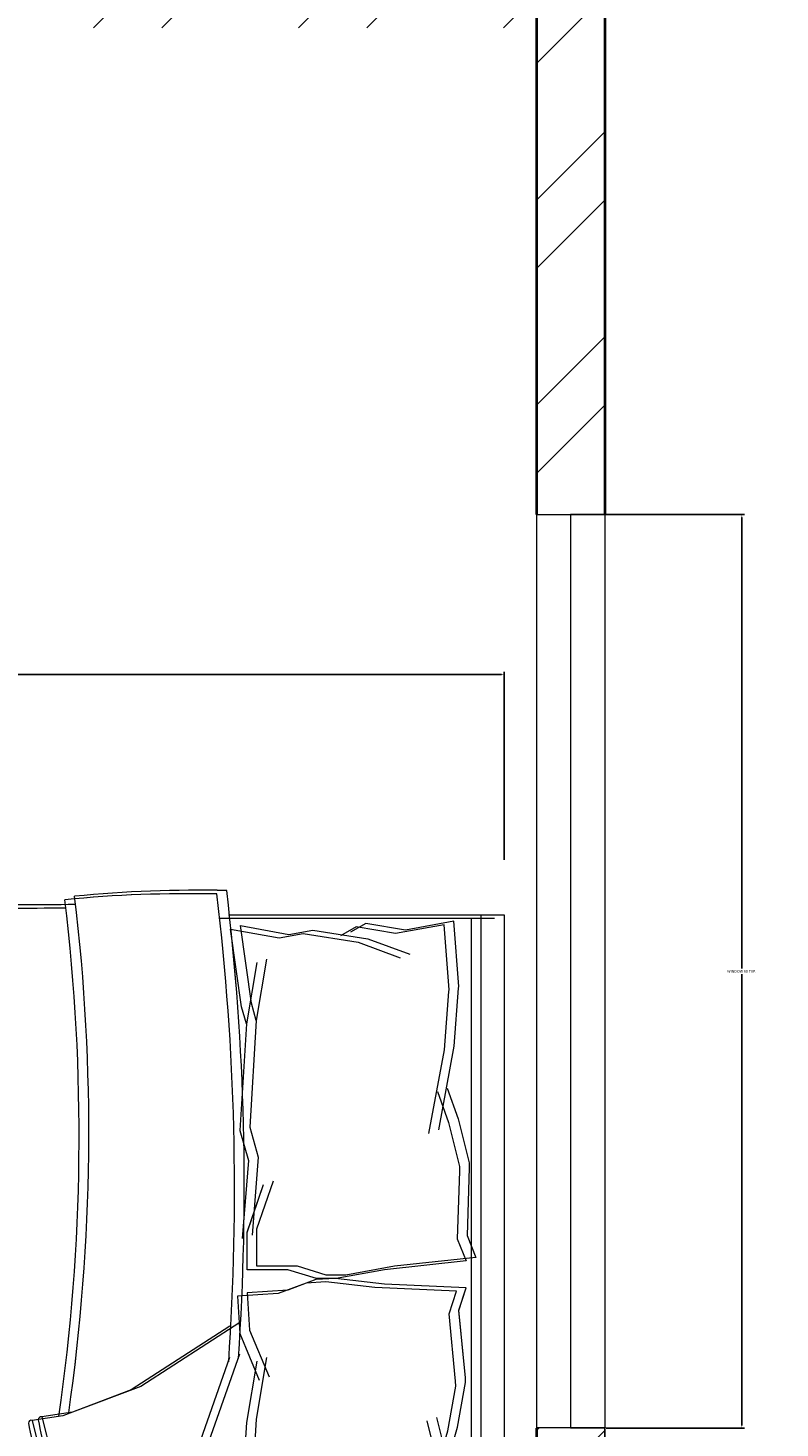
# Model space of a CAD drawing. Units: inches. Extents: x 1601 to 2297, y 1496 to 2631.
# Tile 22 of 57: x 2193 to 2242, y 1701 to 1793. Entities that reach past the tile are written whole.
import ezdxf

# ---------------------------------------------------------------- set-up
doc = ezdxf.new("R2010")
doc.units = ezdxf.units.IN
for name, color, linetype, lineweight in [('A-ANNO-DIMS', 2, 'Continuous', 18), ('A-FURN', 8, 'Continuous', 18), ('A-GLAZ', 161, 'Continuous', 20), ('A-WALL', 7, 'Continuous', 40), ('A-WALL-PATT', 215, 'Continuous', 13)]:
    doc.layers.add(name, color=color, linetype=linetype, lineweight=lineweight)
doc.styles.get("Standard").update_dxf_attribs({"font": 'arial.ttf'})
doc.dimstyles.get("Standard").update_dxf_attribs({"dimtxt": 0.18, "dimasz": 0.18, "dimexe": 0.18, "dimexo": 0.0625, "dimgap": 0.09, "dimtad": 0, "dimtih": 1, "dimtoh": 1, "dimdec": 4, "dimzin": 0, "dimdsep": 46, "dimtxsty": 'Standard', "dimcen": 0.09, "dimadec": 0, "dimazin": 0, "dimtfac": 1, "dimtdec": 4, "dimtofl": 0, "dimtmove": 0, "dimatfit": 3, "dimfxl": 1, "dimtolj": 1, "dimtzin": 0, "dimarcsym": 0})

# ---------------------------------------------------------------- blocks, each defined once
blk = doc.blocks.new('BED-DOUBLE')
for p, q in [((27.746, 52.867), (24.495, 49.162)), ((27.746, 52.867), (24.495, 49.162)), ((27.746, 52.867), (24.495, 49.162)), ((27.746, 52.867), (24.495, 49.162)), ((28.385, 53.096), (25.135, 49.39)), ((28.385, 53.096), (25.135, 49.39)), ((28.385, 53.096), (25.135, 49.39)), ((28.385, 53.096), (25.135, 49.39)), ((29.49, 52.947), (27.746, 52.867, 3.871)), ((29.49, 52.947), (27.746, 52.867, 3.871)), ((29.49, 52.947), (27.746, 52.867, 3.871)), ((29.49, 52.947), (27.746, 52.867, 3.871)), ((28.365, 51.33), (27.746, 52.867)), ((28.365, 51.33), (27.746, 52.867)), ((28.365, 51.33), (27.746, 52.867)), ((28.365, 51.33), (27.746, 52.867)), ((30.13, 53.175), (28.385, 53.096, 3.871)), ((30.13, 53.175), (28.385, 53.096, 3.871)), ((30.13, 53.175), (28.385, 53.096, 3.871)), ((30.13, 53.175), (28.385, 53.096, 3.871)), ((29.004, 51.559), (28.385, 53.096)), ((29.004, 51.558), (28.385, 53.096)), ((29.004, 51.559), (28.385, 53.096)), ((29.004, 51.558), (28.385, 53.096)), ((28.695, 48.461), (29.004, 51.559)), ((28.695, 48.461), (29.004, 51.559)), ((28.695, 48.461), (29.004, 51.558)), ((28.695, 48.461), (29.004, 51.558)), ((0, 51.494), (0.639, 51.493)), ((0, 3.475), (0, 51.494)), ((0, 51.494), (0.639, 51.493)), ((0, 3.475), (0, 51.494)), ((0, 51.265), (26.61, 51.265)), ((0, 51.265), (26.61, 51.265)), ((0, 51.265), (26.61, 51.265)), ((0, 51.265), (26.61, 51.265)), ((0.639, 51.494), (27.249, 51.494)), ((0.639, 51.494), (27.249, 51.494)), ((0.639, 51.493), (27.249, 51.493)), ((0.639, 51.493), (27.249, 51.493)), ((1.533, 3.475), (1.533, 51.265)), ((1.533, 3.475), (1.533, 51.265)), ((1.533, 3.475), (1.533, 51.265)), ((1.533, 3.475), (1.533, 51.265)), ((2.173, 3.703), (2.173, 51.494)), ((2.173, 3.703), (2.173, 51.494)), ((2.173, 3.703), (2.173, 51.493)), ((2.173, 3.703), (2.173, 51.493)), ((16.573, 50.698), (13.434, 49.923)), ((16.573, 50.698), (13.434, 49.922)), ((16.573, 50.698), (13.434, 49.923)), ((16.573, 50.698), (13.434, 49.922)), ((17.212, 50.926), (14.073, 50.151)), ((17.212, 50.926), (14.073, 50.151)), ((17.212, 50.926), (14.073, 50.151)), ((17.212, 50.926), (14.073, 50.151)), ((16.169, 45.566), (16.573, 50.698)), ((16.169, 45.566), (16.573, 50.698)), ((16.169, 45.566), (16.573, 50.698)), ((16.169, 45.566), (16.573, 50.698)), ((16.808, 45.795), (17.212, 50.926)), ((16.808, 45.794), (17.212, 50.926)), ((16.808, 45.795), (17.212, 50.926)), ((16.808, 45.794), (17.212, 50.926)), ((28.055, 48.233), (28.365, 51.33)), ((28.055, 48.233), (28.365, 51.33)), ((28.055, 48.233), (28.365, 51.33)), ((28.055, 48.233), (28.365, 51.33)), ((2.557, 50.112), (2.46, 44.709)), ((2.557, 50.112), (2.46, 44.709)), ((2.557, 50.111), (2.46, 44.709)), ((2.557, 50.111), (2.46, 44.709)), ((2.557, 50.112), (5.768, 49.733)), ((2.557, 50.112), (5.768, 49.733)), ((2.557, 50.111), (5.768, 49.733)), ((2.557, 50.111), (5.768, 49.733)), ((3.196, 50.34), (3.099, 44.938)), ((3.196, 50.34), (3.099, 44.938)), ((3.196, 50.34), (3.099, 44.938)), ((3.196, 50.34), (3.099, 44.938)), ((3.196, 50.34), (6.407, 49.961)), ((3.196, 50.34), (6.407, 49.961)), ((3.196, 50.34), (6.407, 49.961)), ((3.196, 50.34), (6.407, 49.961)), ((5.768, 49.733), (8.338, 50.328)), ((5.768, 49.733), (8.338, 50.328)), ((5.768, 49.733), (8.338, 50.328)), ((5.768, 49.733), (8.338, 50.328)), ((6.407, 49.961), (8.977, 50.557)), ((6.407, 49.961), (8.977, 50.557)), ((6.407, 49.961), (8.977, 50.556)), ((6.407, 49.961), (8.977, 50.556)), ((11.829, 50.112), (8.257, 49.309)), ((11.829, 50.112), (8.257, 49.309)), ((11.829, 50.112), (8.257, 49.309)), ((11.829, 50.112), (8.257, 49.309)), ((8.338, 50.328), (9.384, 49.814)), ((8.338, 50.328), (9.384, 49.814)), ((8.338, 50.328), (9.384, 49.814)), ((8.338, 50.328), (9.384, 49.814)), ((12.468, 50.34), (8.896, 49.538)), ((12.468, 50.34), (8.896, 49.537)), ((12.468, 50.34), (8.896, 49.538)), ((12.468, 50.34), (8.896, 49.537)), ((8.977, 50.557), (10.024, 50.043)), ((8.977, 50.557), (10.024, 50.043)), ((8.977, 50.556), (10.024, 50.042)), ((8.977, 50.556), (10.024, 50.042)), ((13.434, 49.923), (11.829, 50.112)), ((13.434, 49.922), (11.829, 50.112)), ((13.434, 49.923), (11.829, 50.112)), ((13.434, 49.922), (11.829, 50.112)), ((14.073, 50.151), (12.468, 50.34)), ((14.073, 50.151), (12.468, 50.34)), ((14.073, 50.151), (12.468, 50.34)), ((14.073, 50.151), (12.468, 50.34)), ((8.257, 49.309), (5.578, 48.128)), ((8.257, 49.309), (5.578, 48.128)), ((8.257, 49.309), (5.578, 48.128)), ((8.257, 49.309), (5.578, 48.128)), ((8.896, 49.538), (6.218, 48.356)), ((8.896, 49.538), (6.218, 48.356)), ((8.896, 49.537), (6.218, 48.356)), ((8.896, 49.537), (6.218, 48.356)), ((24.495, 49.162), (22.329, 46.219)), ((24.495, 49.162), (22.329, 46.219)), ((24.495, 49.162), (22.329, 46.219)), ((24.495, 49.162), (22.329, 46.219)), ((25.135, 49.39), (22.968, 46.448)), ((25.135, 49.39), (22.968, 46.448)), ((25.135, 49.39), (22.968, 46.448)), ((25.135, 49.39), (22.968, 46.448)), ((28.365, 44.361), (28.055, 48.233)), ((28.365, 44.361), (28.055, 48.233)), ((28.365, 44.361), (28.055, 48.233)), ((28.365, 44.361), (28.055, 48.233)), ((29.004, 44.589), (28.695, 48.461)), ((29.004, 44.589), (28.695, 48.461)), ((29.004, 44.589), (28.695, 48.461)), ((29.004, 44.589), (28.695, 48.461)), ((22.329, 46.219), (20.316, 40.644)), ((22.329, 46.219), (20.316, 40.644)), ((22.329, 46.219), (20.317, 40.644)), ((22.329, 46.219), (20.317, 40.644)), ((22.968, 46.448), (20.956, 40.872)), ((22.968, 46.448), (20.956, 40.872)), ((22.968, 46.448), (20.956, 40.872)), ((22.968, 46.448), (20.956, 40.872)), ((2.46, 44.709), (2.542, 45.712)), ((2.46, 44.709), (2.542, 45.712)), ((2.46, 44.709), (2.542, 45.712)), ((2.46, 44.709), (2.542, 45.712)), ((2.542, 45.712), (3.069, 41.914)), ((2.542, 45.712), (3.069, 41.914)), ((2.542, 45.712), (3.069, 41.914)), ((2.542, 45.712), (3.069, 41.914)), ((3.099, 44.938), (3.181, 45.941)), ((3.099, 44.938), (3.181, 45.941)), ((3.099, 44.938), (3.181, 45.94)), ((3.099, 44.938), (3.181, 45.94)), ((3.181, 45.941), (3.709, 42.143)), ((3.181, 45.941), (3.709, 42.143)), ((3.181, 45.94), (3.709, 42.142)), ((3.181, 45.94), (3.709, 42.142)), ((16.726, 43.606), (16.169, 45.566)), ((16.726, 43.606), (16.169, 45.566)), ((16.726, 43.606), (16.169, 45.566)), ((16.726, 43.606), (16.169, 45.566)), ((17.365, 43.834), (16.808, 45.795)), ((17.365, 43.834), (16.808, 45.795)), ((17.365, 43.834), (16.808, 45.794)), ((17.365, 43.834), (16.808, 45.794)), ((28.829, 40.954), (28.365, 44.361)), ((28.829, 40.953), (28.365, 44.361)), ((28.829, 40.954), (28.365, 44.361)), ((28.829, 40.953), (28.365, 44.361)), ((29.468, 41.182), (29.004, 44.589)), ((29.469, 41.182), (29.004, 44.589)), ((29.468, 41.182), (29.004, 44.589)), ((29.469, 41.182), (29.004, 44.589)), ((16.295, 36.596), (16.726, 43.606)), ((16.295, 36.596), (16.726, 43.606)), ((16.295, 36.596), (16.726, 43.606)), ((16.295, 36.596), (16.726, 43.606)), ((16.934, 36.824), (17.365, 43.834)), ((16.934, 36.824), (17.365, 43.834)), ((16.934, 36.824), (17.365, 43.834)), ((16.934, 36.824), (17.365, 43.834)), ((3.069, 41.914), (4.422, 36.495)), ((3.069, 41.914), (4.422, 36.495)), ((3.069, 41.914), (4.422, 36.495)), ((3.069, 41.914), (4.422, 36.495)), ((3.709, 42.143), (5.061, 36.723)), ((3.709, 42.143), (5.061, 36.723)), ((3.709, 42.142), (5.061, 36.723)), ((3.709, 42.142), (5.061, 36.723)), ((20.316, 40.644), (17.383, 32.306)), ((20.317, 40.644), (17.383, 32.306)), ((20.316, 40.644), (17.383, 32.306)), ((20.317, 40.644), (17.383, 32.306)), ((20.956, 40.872), (18.022, 32.534)), ((20.956, 40.872), (18.022, 32.534)), ((20.956, 40.872), (18.022, 32.534)), ((20.956, 40.872), (18.022, 32.534)), ((29.758, 38.94), (28.829, 40.954)), ((29.758, 38.94), (28.829, 40.954)), ((29.758, 38.94), (28.829, 40.953)), ((29.758, 38.94), (28.829, 40.953)), ((30.397, 39.169), (29.468, 41.182)), ((30.397, 39.169), (29.468, 41.182)), ((30.397, 39.168), (29.469, 41.182)), ((30.397, 39.168), (29.469, 41.182)), ((79.245, 15.063), (79.245, 39.677)), ((79.245, 15.063), (79.245, 39.677)), ((79.245, 15.063), (79.245, 39.677)), ((79.245, 15.063), (79.245, 39.677)), ((79.884, 15.292), (79.884, 39.905)), ((79.884, 15.291), (79.884, 39.905)), ((79.884, 15.292), (79.884, 39.905)), ((79.884, 15.291), (79.884, 39.905)), ((3.673, 39.2), (3.078, 37.135)), ((3.673, 39.2), (3.078, 37.135)), ((3.673, 39.2), (3.078, 37.135)), ((3.673, 39.2), (3.078, 37.135)), ((4.313, 39.428), (3.717, 37.363)), ((4.313, 39.428), (3.717, 37.363)), ((4.313, 39.428), (3.718, 37.363)), ((4.313, 39.428), (3.718, 37.363)), ((30.377, 36.462), (29.758, 38.94)), ((30.377, 36.462), (29.758, 38.94)), ((30.377, 36.462), (29.758, 38.94)), ((30.377, 36.462), (29.758, 38.94)), ((31.016, 36.691), (30.397, 39.169)), ((31.016, 36.691), (30.397, 39.169)), ((31.016, 36.691), (30.397, 39.168)), ((31.016, 36.691), (30.397, 39.168)), ((3.078, 37.135), (2.537, 34.204)), ((3.078, 37.135), (2.537, 34.204)), ((3.078, 37.135), (2.537, 34.204)), ((3.078, 37.135), (2.537, 34.204)), ((3.717, 37.363), (3.176, 34.433)), ((3.718, 37.363), (3.176, 34.433)), ((3.717, 37.363), (3.176, 34.433)), ((3.718, 37.363), (3.176, 34.433)), ((16.268, 32.792), (16.934, 36.824)), ((16.268, 32.792), (16.934, 36.824)), ((16.268, 32.792), (16.934, 36.824)), ((16.268, 32.792), (16.934, 36.824)), ((15.628, 32.564), (16.295, 36.596)), ((15.628, 32.564), (16.295, 36.596)), ((15.628, 32.564), (16.295, 36.596)), ((15.628, 32.564), (16.295, 36.596)), ((23.876, 34.449), (28.365, 36.153)), ((23.876, 34.449), (28.365, 36.153)), ((23.876, 34.449), (28.365, 36.152)), ((23.876, 34.449), (28.365, 36.152)), ((24.516, 34.677), (29.004, 36.381)), ((24.516, 34.677), (29.004, 36.381)), ((24.516, 34.677), (29.004, 36.381)), ((24.516, 34.677), (29.004, 36.381)), ((28.365, 36.153), (30.377, 36.462)), ((28.365, 36.152), (30.377, 36.462)), ((28.365, 36.153), (30.377, 36.462)), ((28.365, 36.152), (30.377, 36.462)), ((29.004, 36.381), (31.016, 36.691)), ((29.004, 36.381), (31.016, 36.691)), ((29.004, 36.381), (31.016, 36.691)), ((29.004, 36.381), (31.016, 36.691)), ((2.537, 34.204), (2.557, 33.883)), ((2.537, 34.204), (2.557, 33.883)), ((2.537, 34.204), (2.557, 33.883)), ((2.537, 34.204), (2.557, 33.883)), ((3.176, 34.433), (3.196, 34.112)), ((3.176, 34.433), (3.196, 34.112)), ((3.176, 34.433), (3.196, 34.112)), ((3.176, 34.433), (3.196, 34.112)), ((3.196, 34.112), (3.618, 29.684)), ((3.196, 34.112), (3.618, 29.684)), ((3.196, 34.112), (3.618, 29.684)), ((3.196, 34.112), (3.618, 29.684)), ((17.379, 30.978), (16.094, 34.049)), ((17.379, 30.978), (16.094, 34.049)), ((17.379, 30.978), (16.094, 34.049)), ((17.379, 30.978), (16.094, 34.049)), ((17.383, 30.259), (23.876, 34.449)), ((17.383, 30.259), (23.876, 34.449)), ((17.383, 30.259), (23.876, 34.449)), ((17.383, 30.259), (23.876, 34.449)), ((18.022, 30.487), (24.516, 34.677)), ((18.022, 30.487), (24.516, 34.677)), ((18.022, 30.487), (24.516, 34.677)), ((18.022, 30.487), (24.516, 34.677)), ((2.557, 33.883), (2.979, 29.456)), ((2.557, 33.883), (2.979, 29.455)), ((2.557, 33.883), (2.979, 29.456)), ((2.557, 33.883), (2.979, 29.455)), ((16.739, 30.75), (15.454, 33.821)), ((16.739, 30.75), (15.454, 33.821)), ((16.739, 30.75), (15.454, 33.82)), ((16.739, 30.75), (15.454, 33.82)), ((16.893, 28.297), (16.739, 30.75)), ((16.893, 28.297), (16.739, 30.75)), ((16.893, 28.297), (16.739, 30.75)), ((16.893, 28.297), (16.739, 30.75)), ((17.532, 28.526), (17.379, 30.978)), ((17.532, 28.525), (17.379, 30.978)), ((17.532, 28.526), (17.379, 30.978)), ((17.532, 28.525), (17.379, 30.978)), ((2.979, 29.456), (2.492, 27.977)), ((2.979, 29.456), (2.492, 27.977)), ((2.979, 29.455), (2.492, 27.976)), ((2.979, 29.455), (2.492, 27.976)), ((3.618, 29.684), (3.131, 28.205)), ((3.618, 29.684), (3.131, 28.205)), ((3.618, 29.684), (3.131, 28.205)), ((3.618, 29.684), (3.131, 28.205)), ((14.856, 28.359), (17.532, 28.526)), ((14.856, 28.359), (17.532, 28.526)), ((14.856, 28.358), (17.532, 28.525)), ((14.856, 28.358), (17.532, 28.525)), ((2.492, 27.977), (7.867, 27.733)), ((2.492, 27.977), (7.867, 27.733)), ((2.492, 27.976), (7.867, 27.733)), ((2.492, 27.976), (7.867, 27.733)), ((3.131, 28.205), (8.506, 27.962)), ((3.131, 28.205), (8.506, 27.961)), ((3.131, 28.205), (8.506, 27.962)), ((3.131, 28.205), (8.506, 27.961)), ((7.867, 27.733), (11.078, 27.355)), ((7.867, 27.733), (11.078, 27.354)), ((7.867, 27.733), (11.078, 27.355)), ((7.867, 27.733), (11.078, 27.354)), ((8.506, 27.962), (11.717, 27.583)), ((8.506, 27.962), (11.717, 27.583)), ((8.506, 27.961), (11.717, 27.583)), ((8.506, 27.961), (11.717, 27.583)), ((11.717, 27.583), (13.016, 27.664)), ((11.717, 27.583), (13.016, 27.664)), ((11.717, 27.583), (13.016, 27.664)), ((11.717, 27.583), (13.016, 27.664)), ((12.377, 27.436), (14.216, 28.13)), ((12.377, 27.436), (14.217, 28.13)), ((12.377, 27.436), (14.216, 28.13)), ((12.377, 27.436), (14.217, 28.13)), ((13.016, 27.664), (14.856, 28.359)), ((13.016, 27.664), (14.856, 28.359)), ((13.016, 27.664), (14.856, 28.358)), ((13.016, 27.664), (14.856, 28.358)), ((14.216, 28.13), (16.893, 28.297)), ((14.216, 28.13), (16.893, 28.297)), ((14.217, 28.13), (16.893, 28.297)), ((14.217, 28.13), (16.893, 28.297)), ((2.509, 26.211), (7.859, 26.789)), ((2.509, 26.21), (7.859, 26.789)), ((2.509, 26.211), (7.859, 26.789)), ((2.509, 26.21), (7.859, 26.789)), ((7.22, 26.561), (10.401, 27.139)), ((7.22, 26.56), (10.401, 27.139)), ((7.22, 26.561), (10.401, 27.139)), ((7.22, 26.56), (10.401, 27.139)), ((7.859, 26.789), (11.04, 27.367)), ((7.859, 26.789), (11.04, 27.367)), ((7.859, 26.789), (11.04, 27.367)), ((7.859, 26.789), (11.04, 27.367)), ((10.401, 27.139), (11.702, 27.139)), ((10.401, 27.139), (11.702, 27.139)), ((10.401, 27.139), (11.702, 27.139)), ((10.401, 27.139), (11.702, 27.139)), ((11.04, 27.367), (12.341, 27.367)), ((11.04, 27.367), (12.341, 27.367)), ((11.04, 27.367), (12.341, 27.367)), ((11.04, 27.367), (12.341, 27.367)), ((11.078, 27.355), (12.377, 27.436)), ((11.078, 27.354), (12.377, 27.436)), ((11.078, 27.355), (12.377, 27.436)), ((11.078, 27.354), (12.377, 27.436)), ((11.702, 27.139), (13.582, 26.561)), ((11.702, 27.139), (13.582, 26.56)), ((11.702, 27.139), (13.582, 26.561)), ((11.702, 27.139), (13.582, 26.56)), ((12.341, 27.367), (14.221, 26.789)), ((12.341, 27.367), (14.221, 26.789)), ((12.341, 27.367), (14.221, 26.789)), ((12.341, 27.367), (14.221, 26.789)), ((14.221, 26.789), (16.902, 26.789)), ((14.221, 26.789), (16.902, 26.789)), ((14.221, 26.789), (16.902, 26.789)), ((14.221, 26.789), (16.902, 26.789)), ((16.902, 26.789), (16.902, 24.332)), ((16.902, 26.789), (16.902, 24.331)), ((16.902, 26.789), (16.902, 24.332)), ((16.902, 26.789), (16.902, 24.331)), ((1.87, 25.982), (7.22, 26.561)), ((1.87, 25.982), (7.22, 26.561)), ((1.87, 25.982), (7.22, 26.56)), ((1.87, 25.982), (7.22, 26.56)), ((2.448, 24.537), (1.87, 25.982)), ((2.448, 24.537), (1.87, 25.982)), ((2.448, 24.537), (1.87, 25.982)), ((2.448, 24.537), (1.87, 25.982)), ((3.088, 24.765), (2.509, 26.211)), ((3.088, 24.765), (2.509, 26.211)), ((3.088, 24.765), (2.509, 26.21)), ((3.088, 24.765), (2.509, 26.21)), ((13.582, 26.561), (16.263, 26.561)), ((13.582, 26.561), (16.263, 26.561)), ((13.582, 26.56), (16.263, 26.56)), ((13.582, 26.56), (16.263, 26.56)), ((16.263, 26.561), (16.263, 24.103)), ((16.263, 26.561), (16.263, 24.103)), ((16.263, 26.56), (16.263, 24.103)), ((16.263, 26.56), (16.263, 24.103)), ((2.304, 20.091), (2.448, 24.537)), ((2.304, 20.091), (2.448, 24.537)), ((2.304, 20.091), (2.448, 24.537)), ((2.304, 20.091), (2.448, 24.537)), ((2.943, 20.32), (3.088, 24.765)), ((2.943, 20.319), (3.088, 24.765)), ((2.943, 20.32), (3.088, 24.765)), ((2.943, 20.319), (3.088, 24.765)), ((16.263, 24.103), (15.172, 20.959)), ((16.263, 24.103), (15.172, 20.958)), ((16.263, 24.103), (15.172, 20.959)), ((16.263, 24.103), (15.172, 20.958)), ((16.902, 24.332), (15.811, 21.187)), ((16.902, 24.332), (15.811, 21.187)), ((16.902, 24.331), (15.811, 21.187)), ((16.902, 24.331), (15.811, 21.187)), ((16.169, 19.384), (16.573, 24.516)), ((16.169, 19.384), (16.573, 24.516)), ((16.169, 19.383), (16.573, 24.515)), ((16.169, 19.383), (16.573, 24.515)), ((16.808, 19.612), (17.212, 24.744)), ((16.808, 19.612), (17.212, 24.744)), ((16.808, 19.612), (17.212, 24.744)), ((16.808, 19.612), (17.212, 24.744)), ((2.943, 19.998), (2.943, 20.32)), ((2.943, 19.998), (2.943, 20.32)), ((2.943, 19.998), (2.943, 20.319)), ((2.943, 19.998), (2.943, 20.319)), ((2.304, 19.77), (2.304, 20.091)), ((2.304, 19.769), (2.304, 20.091)), ((2.304, 19.77), (2.304, 20.091)), ((2.304, 19.769), (2.304, 20.091)), ((3.027, 16.878), (2.304, 19.77)), ((3.027, 16.878), (2.304, 19.77)), ((3.027, 16.878), (2.304, 19.769)), ((3.027, 16.878), (2.304, 19.769)), ((3.666, 17.107), (2.943, 19.998)), ((3.666, 17.107), (2.943, 19.998)), ((3.666, 17.107), (2.943, 19.998)), ((3.666, 17.107), (2.943, 19.998)), ((16.726, 17.423), (16.169, 19.384)), ((16.726, 17.423), (16.169, 19.384)), ((16.726, 17.423), (16.169, 19.383)), ((16.726, 17.423), (16.169, 19.383)), ((17.365, 17.652), (16.808, 19.612)), ((17.365, 17.651), (16.808, 19.612)), ((17.365, 17.652), (16.808, 19.612)), ((17.365, 17.651), (16.808, 19.612)), ((3.316, 12.108), (4.328, 17.601)), ((3.316, 12.108), (4.328, 17.601)), ((3.316, 12.108), (4.328, 17.601)), ((3.316, 12.108), (4.328, 17.601)), ((3.955, 12.336), (4.967, 17.83)), ((3.955, 12.336), (4.967, 17.83)), ((3.955, 12.336), (4.967, 17.829)), ((3.955, 12.336), (4.967, 17.829)), ((16.934, 10.642), (17.365, 17.652)), ((16.934, 10.642), (17.365, 17.652)), ((16.934, 10.642), (17.365, 17.651)), ((16.934, 10.642), (17.365, 17.651)), ((3.75, 14.855), (3.027, 16.878)), ((3.75, 14.854), (3.027, 16.878)), ((3.75, 14.855), (3.027, 16.878)), ((3.75, 14.854), (3.027, 16.878)), ((4.389, 15.083), (3.666, 17.107)), ((4.389, 15.083), (3.666, 17.107)), ((4.389, 15.083), (3.666, 17.107)), ((4.389, 15.083), (3.666, 17.107)), ((16.295, 10.413), (16.726, 17.423)), ((16.295, 10.413), (16.726, 17.423)), ((16.295, 10.413), (16.726, 17.423)), ((16.295, 10.413), (16.726, 17.423)), ((3.027, 8.285), (3.316, 12.108)), ((3.027, 8.284), (3.316, 12.108)), ((3.027, 8.285), (3.316, 12.108)), ((3.027, 8.284), (3.316, 12.108)), ((3.666, 8.513), (3.955, 12.336)), ((3.666, 8.513), (3.955, 12.336)), ((3.666, 8.513), (3.955, 12.336)), ((3.666, 8.513), (3.955, 12.336)), ((15.628, 6.382), (16.295, 10.413)), ((15.628, 6.381), (16.295, 10.413)), ((15.628, 6.382), (16.295, 10.413)), ((15.628, 6.381), (16.295, 10.413)), ((16.268, 6.61), (16.934, 10.642)), ((16.268, 6.61), (16.934, 10.642)), ((16.268, 6.61), (16.934, 10.642)), ((16.268, 6.61), (16.934, 10.642)), ((16.295, 10.413), (16.618, 9.28)), ((16.295, 10.413), (16.618, 9.28)), ((16.295, 10.413), (16.618, 9.28)), ((16.295, 10.413), (16.618, 9.28)), ((16.934, 10.642), (17.257, 9.509)), ((16.934, 10.642), (17.257, 9.508)), ((16.934, 10.642), (17.257, 9.509)), ((16.934, 10.642), (17.257, 9.508)), ((16.618, 9.28), (17.341, 4.184)), ((16.618, 9.28), (17.341, 4.183)), ((16.618, 9.28), (17.341, 4.184)), ((16.618, 9.28), (17.341, 4.183)), ((17.257, 9.509), (17.98, 4.412)), ((17.257, 9.509), (17.98, 4.412)), ((17.257, 9.508), (17.98, 4.412)), ((17.257, 9.508), (17.98, 4.412)), ((3.009, 8.179), (3.027, 8.285)), ((3.009, 8.179), (3.027, 8.285)), ((3.009, 8.179), (3.027, 8.284)), ((3.009, 8.179), (3.027, 8.284)), ((3.648, 8.408), (3.666, 8.513)), ((3.648, 8.407), (3.666, 8.513)), ((3.648, 8.408), (3.666, 8.513)), ((3.648, 8.407), (3.666, 8.513)), ((3.977, 4.127), (3.648, 8.408)), ((3.977, 4.127), (3.648, 8.408)), ((3.977, 4.127), (3.648, 8.407)), ((3.977, 4.127), (3.648, 8.407)), ((3.338, 3.898), (3.009, 8.179)), ((3.338, 3.898), (3.009, 8.179)), ((3.338, 3.898), (3.009, 8.179)), ((3.338, 3.898), (3.009, 8.179)), ((8.955, 5.051), (6.208, 6.063)), ((8.955, 5.051), (6.208, 6.063)), ((8.955, 5.051), (6.208, 6.063)), ((8.955, 5.051), (6.208, 6.063)), ((9.594, 5.279), (6.847, 6.291)), ((9.594, 5.279), (6.847, 6.291)), ((9.594, 5.279), (6.847, 6.291)), ((9.594, 5.279), (6.847, 6.291)), ((3.955, 4.123), (7.136, 4.701)), ((3.955, 4.123), (7.136, 4.701)), ((3.955, 4.123), (7.136, 4.701)), ((3.955, 4.123), (7.136, 4.701)), ((7.136, 4.701), (9.739, 4.267)), ((7.136, 4.701), (9.739, 4.267)), ((7.136, 4.701), (9.739, 4.267)), ((7.136, 4.701), (9.739, 4.267)), ((12.57, 4.473), (8.955, 5.051)), ((12.57, 4.472), (8.955, 5.051)), ((12.57, 4.473), (8.955, 5.051)), ((12.57, 4.472), (8.955, 5.051)), ((9.099, 4.039), (10.112, 4.617)), ((9.099, 4.039), (10.112, 4.617)), ((9.099, 4.039), (10.112, 4.617)), ((9.099, 4.039), (10.112, 4.617)), ((13.209, 4.701), (9.594, 5.279)), ((13.209, 4.701), (9.594, 5.279)), ((13.209, 4.701), (9.594, 5.279)), ((13.209, 4.701), (9.594, 5.279)), ((9.739, 4.267), (10.751, 4.846)), ((9.739, 4.267), (10.751, 4.846)), ((9.739, 4.267), (10.751, 4.845)), ((9.739, 4.267), (10.751, 4.845)), ((14.16, 4.762), (12.57, 4.473)), ((14.16, 4.762), (12.57, 4.472)), ((14.16, 4.762), (12.57, 4.473)), ((14.16, 4.762), (12.57, 4.472)), ((14.799, 4.99), (13.209, 4.701)), ((14.799, 4.99), (13.209, 4.701)), ((14.799, 4.99), (13.209, 4.701)), ((14.799, 4.99), (13.209, 4.701)), ((17.341, 4.184), (14.16, 4.762)), ((17.341, 4.183), (14.16, 4.762)), ((17.341, 4.184), (14.16, 4.762)), ((17.341, 4.183), (14.16, 4.762)), ((17.98, 4.412), (14.799, 4.99)), ((17.98, 4.412), (14.799, 4.99)), ((17.98, 4.412), (14.799, 4.99)), ((17.98, 4.412), (14.799, 4.99)), ((18.75, 3.703), (0.639, 3.703)), ((18.75, 3.703), (0.639, 3.703)), ((18.75, 3.703), (0.639, 3.703)), ((18.75, 3.703), (0.639, 3.703)), ((3.316, 3.894), (6.497, 4.473)), ((3.316, 3.894), (6.497, 4.473)), ((3.316, 3.894), (6.497, 4.472)), ((3.316, 3.894), (6.497, 4.472)), ((6.497, 4.473), (9.099, 4.039)), ((6.497, 4.473), (9.099, 4.039)), ((6.497, 4.472), (9.099, 4.039)), ((6.497, 4.472), (9.099, 4.039)), ((18.11, 3.475), (0, 3.475)), ((18.11, 3.475), (0, 3.475)), ((18.11, 3.475), (0, 3.475)), ((18.11, 3.475), (0, 3.475))]:
    blk.add_line(p, q)
for centre, radius, start, end in [((68.666, 76.157), 23.065, 267.47136, 296.46809), ((68.666, 76.157), 23.065, 267.47136, 296.46809), ((68.666, 76.157), 23.065, 267.47136, 296.46809), ((68.666, 76.157), 23.065, 267.47136, 296.46809), ((69.306, 76.385), 23.065, 267.47136, 296.46809), ((69.306, 76.385), 23.065, 267.47136, 296.46809), ((69.306, 76.385), 23.065, 267.47136, 296.46809), ((69.306, 76.385), 23.065, 267.47136, 296.46809), ((78.87, 54.41), 1.102, 332.65876, 86.02002), ((78.87, 54.409), 1.102, 332.65876, 86.02002), ((78.87, 54.41), 1.102, 332.65876, 86.02002), ((78.87, 54.409), 1.102, 332.65876, 86.02002), ((79.509, 54.638), 1.102, 332.65876, 86.02002), ((79.509, 54.638), 1.102, 332.65876, 86.02002), ((79.509, 54.638), 1.102, 332.65876, 86.02002), ((79.509, 54.638), 1.102, 332.65876, 86.02002), ((68.461, -4508.515), 4561.858, 90.002168, 90.286887), ((68.461, -4508.515), 4561.858, 90.002168, 90.286887), ((68.461, -4508.516), 4561.858, 90.002168, 90.286887), ((68.461, -4508.516), 4561.858, 90.002168, 90.286887), ((212.276, 41.152), 133.04, 174.4998, 180.63509), ((212.277, 41.151), 133.04, 174.4998, 180.63509), ((212.276, 41.152), 133.04, 174.4998, 180.63509), ((212.277, 41.151), 133.04, 174.4998, 180.63509), ((212.916, 41.38), 133.04, 174.4998, 180.63509), ((212.916, 41.38), 133.04, 174.4998, 180.63509), ((212.916, 41.38), 133.04, 174.4998, 180.63509), ((212.916, 41.38), 133.04, 174.4998, 180.63509), ((-6.656, 51.327), 36.183, 349.87628, 2.56571), ((-6.656, 51.327), 36.183, 349.87628, 2.56571), ((-6.656, 51.327), 36.183, 349.87628, 2.56571), ((-6.656, 51.327), 36.183, 349.87628, 2.56571), ((36.315, 182.266), 129.499, 266.97912, 273.83645), ((36.315, 182.265), 129.499, 266.97912, 273.83645), ((36.315, 182.266), 129.499, 266.97912, 273.83645), ((36.315, 182.265), 129.499, 266.97912, 273.83645), ((-6.017, 51.555), 36.183, 349.87628, 2.56571), ((-6.017, 51.555), 36.183, 349.87628, 2.56571), ((-6.017, 51.555), 36.183, 349.87628, 2.56571), ((-6.017, 51.555), 36.183, 349.87628, 2.56571), ((36.954, 182.494), 129.499, 266.97912, 273.83645), ((36.954, 182.494), 129.499, 266.97912, 273.83645), ((36.954, 182.494), 129.499, 266.97912, 273.83645), ((36.954, 182.494), 129.499, 266.97912, 273.83645), ((67.821, -4508.744), 4561.858, 90.002168, 90.286887), ((67.821, -4508.744), 4561.858, 90.002168, 90.286887), ((67.821, -4508.744), 4561.858, 90.002168, 90.286887), ((67.821, -4508.744), 4561.858, 90.002168, 90.286887), ((35.705, 43.972), 6.224, 168.6608, 203.73842), ((35.705, 43.971), 6.224, 168.6608, 203.73842), ((35.705, 43.972), 6.224, 168.6608, 203.73842), ((35.705, 43.971), 6.224, 168.6608, 203.73842), ((35.066, 43.743), 6.224, 168.6608, 203.73842), ((35.066, 43.743), 6.224, 168.6608, 203.73842), ((35.066, 43.743), 6.224, 168.6608, 203.73842), ((35.066, 43.743), 6.224, 168.6608, 203.73842), ((2.121, 31.382), 29.654, 10.66171, 19.88058), ((2.121, 31.382), 29.654, 10.66171, 19.88058), ((2.121, 31.382), 29.654, 10.66171, 19.88058), ((2.121, 31.382), 29.654, 10.66171, 19.88058), ((1.482, 31.154), 29.654, 10.66171, 19.88058), ((1.482, 31.154), 29.654, 10.66171, 19.88058), ((1.482, 31.153), 29.654, 10.66171, 19.88058), ((1.482, 31.153), 29.654, 10.66171, 19.88058), ((31.079, 36.864), 0.185, 250.24637, 1.13765), ((31.079, 36.864), 0.185, 250.24637, 1.13765), ((31.079, 36.864), 0.185, 250.24637, 1.13765), ((31.079, 36.864), 0.185, 250.24637, 1.13765), ((156.316, 17.756), 129.02, 171.78449, 186.90062), ((156.316, 17.755), 129.02, 171.78449, 186.90062), ((156.316, 17.756), 129.02, 171.78449, 186.90062), ((156.316, 17.755), 129.02, 171.78449, 186.90062), ((156.955, 17.984), 129.02, 171.78449, 186.90062), ((156.955, 17.984), 129.02, 171.78449, 186.90062), ((156.955, 17.984), 129.02, 171.78449, 186.90062), ((156.955, 17.984), 129.02, 171.78449, 186.90062), ((30.439, 36.636), 0.185, 250.24637, 1.13765), ((30.439, 36.636), 0.185, 250.24637, 1.13765), ((30.439, 36.636), 0.185, 250.24637, 1.13765), ((30.439, 36.636), 0.185, 250.24637, 1.13765), ((182.052, 21.359), 164.969, 176.08655, 186.78213), ((182.052, 21.359), 164.969, 176.08655, 186.78213), ((182.052, 21.358), 164.969, 176.08655, 186.78213), ((182.052, 21.358), 164.969, 176.08655, 186.78213), ((182.692, 21.587), 164.969, 176.08655, 186.78213), ((182.692, 21.587), 164.969, 176.08655, 186.78213), ((182.692, 21.587), 164.969, 176.08655, 186.78213), ((182.692, 21.587), 164.969, 176.08655, 186.78213), ((-23.712, -17.222), 106.459, 13.38322, 17.70533), ((-23.712, -17.222), 106.459, 13.38322, 17.70533), ((-23.712, -17.222), 106.459, 13.38322, 17.70533), ((-23.712, -17.222), 106.459, 13.38322, 17.70533), ((-23.073, -16.994), 106.459, 13.38322, 17.70533), ((-23.073, -16.994), 106.459, 13.38322, 17.70533), ((-23.073, -16.994), 106.459, 13.38322, 17.70533), ((-23.073, -16.994), 106.459, 13.38322, 17.70533), ((200.837, 21.427), 121.759, 182.99578, 189.40907), ((200.837, 21.426), 121.759, 182.99578, 189.40907), ((200.837, 21.427), 121.759, 182.99578, 189.40907), ((200.837, 21.426), 121.759, 182.99578, 189.40907), ((201.476, 21.655), 121.759, 182.99578, 189.40907), ((201.476, 21.655), 121.759, 182.99578, 189.40907), ((201.476, 21.655), 121.759, 182.99578, 189.40907), ((201.476, 21.655), 121.759, 182.99578, 189.40907), ((31.174, -167.308), 170.11, 88.4762, 91.00819), ((31.174, -167.308), 170.11, 88.4762, 91.00819), ((31.174, -167.308), 170.11, 88.4762, 91.00819), ((31.174, -167.308), 170.11, 88.4762, 91.00819), ((31.813, -167.079), 170.11, 88.4762, 91.00819), ((31.813, -167.08), 170.11, 88.4762, 91.00819), ((31.813, -167.079), 170.11, 88.4762, 91.00819), ((31.813, -167.08), 170.11, 88.4762, 91.00819), ((51.253, 485.051), 482.31, 268.22771, 271.71854), ((51.253, 485.05), 482.31, 268.22771, 271.71854), ((51.253, 485.051), 482.31, 268.22771, 271.71854), ((51.253, 485.05), 482.31, 268.22771, 271.71854), ((65.154, -26.671), 29.634, 76.06484, 88.91125), ((65.154, -26.672), 29.634, 76.06484, 88.91125), ((65.154, -26.671), 29.634, 76.06484, 88.91125), ((65.154, -26.672), 29.634, 76.06484, 88.91125), ((20.096, 85.162), 83.306, 268.72178, 275.60397), ((20.096, 85.161), 83.306, 268.72178, 275.60397), ((20.096, 85.162), 83.306, 268.72178, 275.60397), ((20.096, 85.161), 83.306, 268.72178, 275.60397), ((20.735, 85.39), 83.306, 268.72178, 275.60397), ((20.735, 85.39), 83.306, 268.72178, 275.60397), ((20.736, 85.39), 83.306, 268.72178, 275.60397), ((20.736, 85.39), 83.306, 268.72178, 275.60397), ((50.614, 484.822), 482.31, 268.22771, 271.71854), ((50.614, 484.822), 482.31, 268.22771, 271.71854), ((50.614, 484.822), 482.31, 268.22771, 271.71854), ((50.614, 484.822), 482.31, 268.22771, 271.71854), ((64.515, -26.9), 29.634, 76.06484, 88.91125), ((64.515, -26.9), 29.634, 76.06484, 88.91125), ((64.515, -26.9), 29.634, 76.06484, 88.91125), ((64.515, -26.9), 29.634, 76.06484, 88.91125), ((70.276, -21.66), 23.562, 67.97508, 86.652), ((70.276, -21.66), 23.562, 67.97508, 86.652), ((70.276, -21.66), 23.562, 67.97508, 86.652), ((70.276, -21.66), 23.562, 67.97508, 86.652), ((70.915, -21.431), 23.562, 67.97508, 86.652), ((70.915, -21.432), 23.562, 67.97508, 86.652), ((70.915, -21.431), 23.562, 67.97508, 86.652), ((70.915, -21.432), 23.562, 67.97508, 86.652), ((79.718, 1.087), 1.089, 236.17358, 23.47814), ((79.718, 1.087), 1.089, 236.17358, 23.47814), ((79.718, 1.087), 1.089, 236.17358, 23.47814), ((79.718, 1.087), 1.089, 236.17358, 23.47814), ((80.357, 1.316), 1.089, 236.17358, 23.47814), ((80.357, 1.316), 1.089, 236.17358, 23.47814), ((80.357, 1.315), 1.089, 236.17358, 23.47814), ((80.357, 1.315), 1.089, 236.17358, 23.47814)]:
    blk.add_arc(centre, radius, start, end)
blk = doc.blocks.new('WIN-60IN-JAMB4P5')
for p, q in [((0, 60), (4.5, 60)), ((0, 60), (0, 0)), ((4.5, 60), (2.25, 60)), ((2.25, 60), (2.25, 0)), ((4.5, 60), (4.5, 0)), ((4.5, 0), (0, 0)), ((2.25, 0), (4.5, 0))]:
    blk.add_line(p, q)
blk = doc.blocks.new('*D12')
at = {"layer": 'A-ANNO-DIMS', "color": 0, "lineweight": -2, "transparency": 16777216}
for p, q in [((2142.379, 1738.191), (2142.379, 1750.54)), ((2142.559, 1750.36), (2181.784, 1750.36)), ((2223.747, 1750.36), (2184.522, 1750.36)), ((2223.927, 1738.191), (2223.927, 1750.54))]:
    blk.add_line(p, q, dxfattribs=at)
at = {"layer": 'A-ANNO-DIMS', "color": 0, "transparency": 16777216}
for points in [[(2142.559, 1750.39), (2142.559, 1750.33), (2142.379, 1750.36)], [(2223.747, 1750.39), (2223.747, 1750.33), (2223.927, 1750.36)]]:
    blk.add_solid(points, dxfattribs=at)
at = {"layer": 'Defpoints', "color": 0, "transparency": 16777216}
for p in [(2142.379, 1750.36), (2142.379, 1738.128), (2223.927, 1738.128)]:
    blk.add_point(p, dxfattribs=at)
at = {"layer": 'A-ANNO-DIMS', "color": 0, "transparency": 16777216, "insert": (2183.153, 1750.36), "char_height": 0.18, "attachment_point": 5}
blk.add_mtext('\\A1;DOUBLE BED 82 TYP.', dxfattribs=at)
blk = doc.blocks.new('*D24')
at = {"layer": 'A-ANNO-DIMS', "color": 0, "lineweight": -2, "transparency": 16777216}
for p, q in [((2230.6, 1760.856), (2239.717, 1760.856)), ((2239.537, 1760.676), (2239.537, 1731.039)), ((2239.537, 1701.036), (2239.537, 1730.673)), ((2230.6, 1700.856), (2239.717, 1700.856))]:
    blk.add_line(p, q, dxfattribs=at)
at = {"layer": 'A-ANNO-DIMS', "color": 0, "transparency": 16777216}
for points in [[(2239.507, 1760.676), (2239.567, 1760.676), (2239.537, 1760.856)], [(2239.507, 1701.036), (2239.567, 1701.036), (2239.537, 1700.856)]]:
    blk.add_solid(points, dxfattribs=at)
at = {"layer": 'Defpoints', "color": 0, "transparency": 16777216}
for p in [(2230.537, 1760.856), (2239.537, 1760.856), (2230.537, 1700.856)]:
    blk.add_point(p, dxfattribs=at)
at = {"layer": 'A-ANNO-DIMS', "color": 0, "transparency": 16777216, "insert": (2239.537, 1730.856), "char_height": 0.18, "attachment_point": 5}
blk.add_mtext('\\A1;WINDOW 60 TYP.', dxfattribs=at)
blk = doc.blocks.new('*D25')
at = {"layer": 'A-ANNO-DIMS', "color": 0, "lineweight": -2, "transparency": 16777216}
for p, q in [((2226.037, 1700.794), (2226.037, 1691.676)), ((2230.537, 1700.794), (2230.537, 1691.676)), ((2226.217, 1691.856), (2227.829, 1691.856)), ((2230.357, 1691.856), (2228.745, 1691.856))]:
    blk.add_line(p, q, dxfattribs=at)
at = {"layer": 'A-ANNO-DIMS', "color": 0, "transparency": 16777216}
for points in [[(2226.217, 1691.886), (2226.217, 1691.826), (2226.037, 1691.856)], [(2230.357, 1691.886), (2230.357, 1691.826), (2230.537, 1691.856)]]:
    blk.add_solid(points, dxfattribs=at)
at = {"layer": 'Defpoints', "color": 0, "transparency": 16777216}
for p in [(2226.037, 1700.856), (2230.537, 1700.856), (2230.537, 1691.856)]:
    blk.add_point(p, dxfattribs=at)
at = {"layer": 'A-ANNO-DIMS', "color": 0, "transparency": 16777216, "insert": (2228.287, 1691.856), "char_height": 0.18, "attachment_point": 5}
blk.add_mtext('\\A1;5 TYP.', dxfattribs=at)
blk = doc.blocks.new('*D29')
at = {"layer": 'A-ANNO-DIMS', "color": 0, "lineweight": -2, "transparency": 16777216}
for p, q in [((2230.6, 2532.325), (2279.267, 2532.325)), ((2279.087, 2532.145), (2279.087, 2084.007)), ((2279.087, 1635.505), (2279.087, 2083.643)), ((2230.6, 1635.325), (2279.267, 1635.325))]:
    blk.add_line(p, q, dxfattribs=at)
at = {"layer": 'A-ANNO-DIMS', "color": 0, "transparency": 16777216}
for points in [[(2279.057, 2532.145), (2279.117, 2532.145), (2279.087, 2532.325)], [(2279.057, 1635.505), (2279.117, 1635.505), (2279.087, 1635.325)]]:
    blk.add_solid(points, dxfattribs=at)
at = {"layer": 'Defpoints', "color": 0, "transparency": 16777216}
for p in [(2230.537, 2532.325), (2279.087, 2532.325), (2230.537, 1635.325)]:
    blk.add_point(p, dxfattribs=at)
at = {"layer": 'A-ANNO-DIMS', "color": 0, "transparency": 16777216, "insert": (2279.087, 2083.825), "char_height": 0.18, "attachment_point": 5}
blk.add_mtext('\\A1;897', dxfattribs=at)

msp = doc.modelspace()

# ---------------------------------------------------------------- hatches: boundary and pattern name
at = {"layer": 'A-WALL-PATT'}
h = msp.add_hatch(dxfattribs=at)
h.set_pattern_fill('ANSI32', color=256)
h.paths.add_polyline_path([(2230.5373, 1861.8254), (2182.5373, 1861.8254), (2182.5373, 1885.3637), (2178.0373, 1885.3637), (2178.0373, 1861.8254), (2166.0373, 1861.8254), (2134.5373, 1861.8254), (2130.0373, 1861.8254), (2130.0373, 1841.4682), (2126.8833, 1841.4682), (2126.8833, 1836.9682), (2130.0373, 1836.9682), (2130.0373, 1822.7302), (2134.5373, 1822.7302), (2134.5373, 1857.3254), (2166.0373, 1857.3254), (2226.0373, 1857.3254), (2226.0373, 1846.1155), (2230.5373, 1846.1155)])
h.paths.add_polyline_path([(2226.0373, 1797.3254), (2134.5373, 1797.3254), (2134.5373, 1800.6636), (2132.2873, 1800.6636), (2130.0373, 1800.6636), (2130.0373, 1797.3254), (2130.0373, 1792.8254), (2167.7264, 1792.8254), (2226.0373, 1792.8254)])
h.paths.add_polyline_path([(2230.5373, 1822.1155), (2226.0373, 1822.1155), (2226.0373, 1760.8563), (2230.5373, 1760.8563)])
h.paths.add_polyline_path([(2230.5373, 1700.8563), (2226.0373, 1700.8563), (2226.0373, 1644.3254), (2140.2517, 1644.3254), (2140.2517, 1635.3254), (2230.5373, 1635.3254)])
h.paths.add_polyline_path([(2080.2517, 1639.8254), (2080.2517, 1644.3254), (2035.5373, 1644.3254), (2035.5373, 1792.8254), (2094.0373, 1792.8254), (2094.0373, 1797.3254), (2094.0373, 1836.9682), (2097.1057, 1836.9682), (2097.1057, 1839.2182), (2097.1057, 1841.4682), (2094.0373, 1841.4682), (2094.0373, 1862.2276), (2089.5373, 1862.2276), (2089.5373, 1797.3254), (2035.5373, 1797.3254), (2035.5373, 1857.3254), (2035.5373, 1885.0916), (2031.0373, 1885.0916), (2031.0373, 1710.3254), (2012.329, 1710.3254), (2012.329, 1701.3254), (2031.0373, 1701.3254), (2031.0373, 1644.3254), (2031.0373, 1635.3254), (2080.2517, 1635.3254)])
h.paths.add_polyline_path([(1836.0373, 1653.2033), (1842.6171, 1653.2033), (1842.6171, 1657.7033), (1842.6171, 1662.2033), (1831.5373, 1662.2033), (1831.5373, 1764.2033), (1835.3881, 1764.2033), (1835.3881, 1766.4533), (1835.3881, 1768.7033), (1831.5373, 1768.7033), (1827.0373, 1768.7033), (1827.0373, 1662.2033), (1827.0373, 1635.3254), (1836.0373, 1635.3254)])
h.paths.add_polyline_path([(1893.0373, 1701.3254), (1907.193, 1701.3254), (1907.193, 1705.8254), (1907.193, 1710.3254), (1893.0373, 1710.3254), (1893.0373, 1819.8254), (1882.6444, 1819.8254), (1882.6444, 1817.5754), (1882.6444, 1815.3254), (1888.5373, 1815.3254), (1888.5373, 1662.2033), (1884.0373, 1662.2033), (1866.6171, 1662.2033), (1866.6171, 1653.2033), (1882.391, 1653.2033), (1884.0373, 1653.2033), (1884.0373, 1635.3254), (1893.0373, 1635.3254)])
h.paths.add_polyline_path([(1739.3335, 1639.8254), (1739.3335, 1644.3254), (1695.0373, 1644.3254), (1695.0373, 1702.0135), (1690.5373, 1702.0135), (1686.0373, 1702.0135), (1686.0373, 1635.3254), (1739.3335, 1635.3254)])
h.paths.add_polyline_path([(1827.0373, 1644.3254), (1799.3335, 1644.3254), (1799.3335, 1635.3254), (1827.0373, 1635.3254)])
h.paths.add_polyline_path([(1695.0373, 1815.3254), (1849.2759, 1815.3254), (1849.2759, 1819.8254), (1807.5373, 1819.8254), (1807.5373, 1879.8254), (1851.1533, 1879.8254), (1851.1533, 1882.0754), (1851.1533, 1884.3254), (1799.3405, 1884.3254), (1799.3405, 1882.0754), (1799.3405, 1879.8254), (1803.0373, 1879.8254), (1803.0373, 1819.8254), (1695.0373, 1819.8254), (1695.0373, 1835.0458), (1690.5373, 1835.0458), (1686.0373, 1835.0458), (1686.0373, 1766.1753), (1695.0373, 1766.1753)])
h.paths.add_polyline_path([(1775.8157, 1884.3254), (1695.0373, 1884.3254), (1695.0373, 1912.9526), (1690.5373, 1912.9526), (1686.0373, 1912.9526), (1686.0373, 1859.0458), (1695.0373, 1859.0458), (1695.0373, 1879.8254), (1775.8157, 1879.8254)])
h.paths.add_polyline_path([(1893.0373, 2031.3254), (1731.5687, 2031.3254), (1731.5687, 2057.4352), (1722.5687, 2057.4352), (1722.5687, 2031.3254), (1686.0373, 2031.3254), (1686.0373, 1972.9526), (1695.0373, 1972.9526), (1695.0373, 2022.3254), (1888.5373, 2022.3254), (1888.5373, 1884.3254), (1883.4996, 1884.3254), (1883.4996, 1879.8254), (1893.0373, 1879.8254), (1893.0373, 1974.3254), (1976.6199, 1974.3254), (1976.6199, 1978.8254), (1968.0373, 1978.8254), (1968.0373, 1983.3254), (1968.0373, 2008.4756), (1963.5373, 2008.4756), (1959.0373, 2008.4756), (1959.0373, 1983.3254), (1893.0373, 1983.3254)])
h.paths.add_polyline_path([(2230.5373, 2140.4745), (2226.0373, 2140.4745), (2226.0373, 2094.3254), (2040.0373, 2094.3254), (2040.0373, 2085.3254), (2178.0373, 2085.3254), (2178.0373, 2065.6965), (2182.5373, 2065.6965), (2182.5373, 2085.3254), (2226.0373, 2085.3254), (2226.0373, 1986.3254), (2211.2679, 1986.3254), (2211.2679, 1981.8254), (2230.5373, 1981.8254)])
h.paths.add_polyline_path([(2187.6292, 1986.3254), (2182.5373, 1986.3254), (2182.5373, 2029.6965), (2178.0373, 2029.6965), (2178.0373, 1986.3254), (2099.05, 1986.3254), (2099.05, 1981.8254), (2178.0373, 1981.8254), (2178.0373, 1969.3637), (2182.5373, 1969.3637), (2182.5373, 1981.8254), (2187.6292, 1981.8254), (2187.6292, 1984.0754)])
h.paths.add_polyline_path([(1807.1169, 1573.5395), (2055.0405, 1573.5395), (2055.0405, 1610.6322), (1807.1169, 1610.6322)], flags=9)
h.paths.add_polyline_path([(1841.1631, 1712.7967), (1870.3957, 1712.7967), (1870.3957, 1731.454), (1841.1631, 1731.454)], flags=9)
h.paths.add_polyline_path([(2144.3862, 1772.185), (2191.0233, 1772.185), (2191.0233, 1790.8423), (2144.3862, 1790.8423)], flags=9)
h.paths.add_polyline_path([(2143.0128, 1827.3312), (2177.9958, 1827.3312), (2177.9958, 1845.9886), (2143.0128, 1845.9886)], flags=25)
h.paths.add_polyline_path([(2041.2439, 1833.5691), (2070.8516, 1833.5691), (2070.8516, 1852.2264), (2041.2439, 1852.2264)], flags=25)
h.paths.add_polyline_path([(2097.2791, 1947.0598), (2134.2061, 1947.0598), (2134.2061, 1965.7171), (2097.2791, 1965.7171)], flags=9)
h.paths.add_polyline_path([(2214.995, 1904.3124), (2214.995, 1942.2899), (2196.3376, 1942.2899), (2196.3376, 1904.3124)], flags=9)
h.paths.add_polyline_path([(2186.6284, 2043.8031), (2219.7935, 2043.8031), (2219.7935, 2062.4605), (2186.6284, 2062.4605)], flags=25)
h.paths.add_polyline_path([(2064.0877, 2031.616), (2097.4949, 2031.616), (2097.4949, 2050.2734), (2064.0877, 2050.2734)], flags=25)
h.paths.add_polyline_path([(1973.1349, 1986.0688), (2008.4009, 1986.0688), (2008.4009, 2004.7261), (1973.1349, 2004.7261)], flags=9)
h.paths.add_polyline_path([(1976.3676, 2106.9635), (2005.7469, 2106.9635), (2005.7469, 2125.6209), (1976.3676, 2125.6209)], flags=9)
h.paths.add_polyline_path([(1991.7852, 2180.4863), (2027.0513, 2180.4863), (2027.0513, 2199.1437), (1991.7852, 2199.1437)], flags=9)
h.paths.add_polyline_path([(2106.1801, 2187.9359), (2152.2101, 2187.9359), (2152.2101, 2206.5932), (2106.1801, 2206.5932)], flags=9)
h.paths.add_polyline_path([(2148.6686, 2262.2542), (2182.318, 2262.2542), (2182.318, 2280.9115), (2148.6686, 2280.9115)], flags=9)
h.paths.add_polyline_path([(2041.6327, 2252.8147), (2071.2405, 2252.8147), (2071.2405, 2271.4721), (2041.6327, 2271.4721)], flags=9)
h.paths.add_polyline_path([(2063.9734, 2375.4265), (2100.9004, 2375.4265), (2100.9004, 2394.0839), (2063.9734, 2394.0839)], flags=9)
h.paths.add_polyline_path([(2216.4955, 2330.9748), (2216.4955, 2370.2654), (2197.8381, 2370.2654), (2197.8381, 2330.9748)], flags=9)
h.paths.add_polyline_path([(2179.1416, 2485.8687), (2212.3067, 2485.8687), (2212.3067, 2504.5261), (2179.1416, 2504.5261)], flags=9)
h.paths.add_polyline_path([(2078.7442, 2471.1516), (2112.1514, 2471.1516), (2112.1514, 2489.809), (2078.7442, 2489.809)], flags=9)
h.paths.add_polyline_path([(1915.9631, 2329.4668), (1952.8902, 2329.4668), (1952.8902, 2348.1241), (1915.9631, 2348.1241)], flags=9)
h.paths.add_polyline_path([(1904.3189, 2499.6709), (1940.4512, 2499.6709), (1940.4512, 2518.3282), (1904.3189, 2518.3282)], flags=9)
h.paths.add_polyline_path([(1892.3665, 2100.4595), (1925.6374, 2100.4595), (1925.6374, 2119.1169), (1892.3665, 2119.1169)], flags=9)
h.paths.add_polyline_path([(1909.2984, 1805.9631), (1946.2254, 1805.9631), (1946.2254, 1824.6205), (1909.2984, 1824.6205)], flags=9)
h.paths.add_polyline_path([(1934.6056, 1658.616), (1970.738, 1658.616), (1970.738, 1677.2733), (1934.6056, 1677.2733)], flags=9)
h.paths.add_polyline_path([(1711.2052, 1789.8902), (1750.0456, 1789.8902), (1750.0456, 1808.5476), (1711.2052, 1808.5476)], flags=25)
h.paths.add_polyline_path([(1742.7874, 1854.6743), (1771.9449, 1854.6743), (1771.9449, 1873.3317), (1742.7874, 1873.3317)], flags=25)
h.paths.add_polyline_path([(1807.3592, 1997.7912), (1850.1116, 1997.7912), (1850.1116, 2016.4486), (1807.3592, 2016.4486)], flags=25)
h.paths.add_polyline_path([(1717.4579, 2237.7844), (1760.2103, 2237.7844), (1760.2103, 2256.4417), (1717.4579, 2256.4417)], flags=9)
h.paths.add_polyline_path([(1780.9285, 2324.0623), (1810.086, 2324.0623), (1810.086, 2342.7197), (1780.9285, 2342.7197)], flags=9)
h.paths.add_polyline_path([(1837.696, 2449.2024), (1866.9286, 2449.2024), (1866.9286, 2467.8598), (1837.696, 2467.8598)], flags=9)
h.paths.add_polyline_path([(1712.7752, 2484.9404), (1751.6156, 2484.9404), (1751.6156, 2503.5977), (1712.7752, 2503.5977)], flags=9)

# ---------------------------------------------------------------- linework, layer by layer
at = {"layer": 'A-WALL'}
for p, q in [((2226.0373, 1822.1155), (2226.0373, 1760.8563)), ((2230.5373, 1822.1155), (2230.5373, 1760.8563)), ((2226.0373, 1700.8563), (2226.0373, 1644.3254))]:
    msp.add_line(p, q, dxfattribs=at)

# ---------------------------------------------------------------- block references
at = {"layer": 'A-FURN', "rotation": 180}
msp.add_blockref('BED-DOUBLE', (2223.9271, 1738.0414), dxfattribs=at)
at = {"layer": 'A-GLAZ'}
msp.add_blockref('WIN-60IN-JAMB4P5', (2226.037, 1700.8568), dxfattribs=at)

# ---------------------------------------------------------------- dimensions: what is measured, and where the dimension line sits
at = {"layer": 'A-ANNO-DIMS'}
dim = msp.add_linear_dim(base=(2279.0873, 2532.3254), p1=(2230.5373, 1635.3254), p2=(2230.5373, 2532.3254), angle=90, dimstyle='Standard', override={"dimdec": 0, "dimlfac": 1, "dimrnd": 0, "dimzin": 0, "dimdsep": 46, "dimlunit": 2}, dxfattribs=at)
dim.commit()
dim.dimension.update_dxf_attribs({"geometry": '*D29', "text_midpoint": (2279.0873, 2083.8254)})
for base, p1, p2, angle, text, picture, middle in [((2239.5373, 1760.8563), (2230.5373, 1700.8563), (2230.5373, 1760.8563), 90, 'WINDOW <> TYP.', '*D24', (2239.5373, 1730.8563)), ((2142.3787, 1750.3604), (2223.9273, 1738.1281), (2142.3787, 1738.1281), 180, 'DOUBLE BED <> TYP.', '*D12', (2183.153, 1750.3604))]:
    dim = msp.add_linear_dim(base=base, p1=p1, p2=p2, angle=angle, text=text, dimstyle='Standard', override={"dimdec": 0, "dimlfac": 1, "dimrnd": 0, "dimzin": 0, "dimdsep": 46, "dimlunit": 2}, dxfattribs=at)
    dim.commit()
    dim.dimension.update_dxf_attribs({"geometry": picture, "text_midpoint": middle})
dim = msp.add_linear_dim(base=(2230.5373150195, 1691.8563063392), p1=(2226.0373150195, 1700.8563063392), p2=(2230.5373150195, 1700.8563063392), text='<> TYP.', dimstyle='Standard', override={"dimdec": 0, "dimlfac": 1, "dimrnd": 0, "dimzin": 0, "dimdsep": 46, "dimlunit": 2}, dxfattribs=at)
dim.commit()
dim.dimension.update_dxf_attribs({"geometry": '*D25', "text_midpoint": (2228.2873150195, 1691.8563063392)})

doc.saveas('drawing.dxf')
